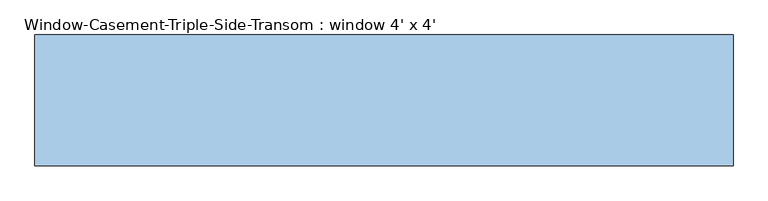
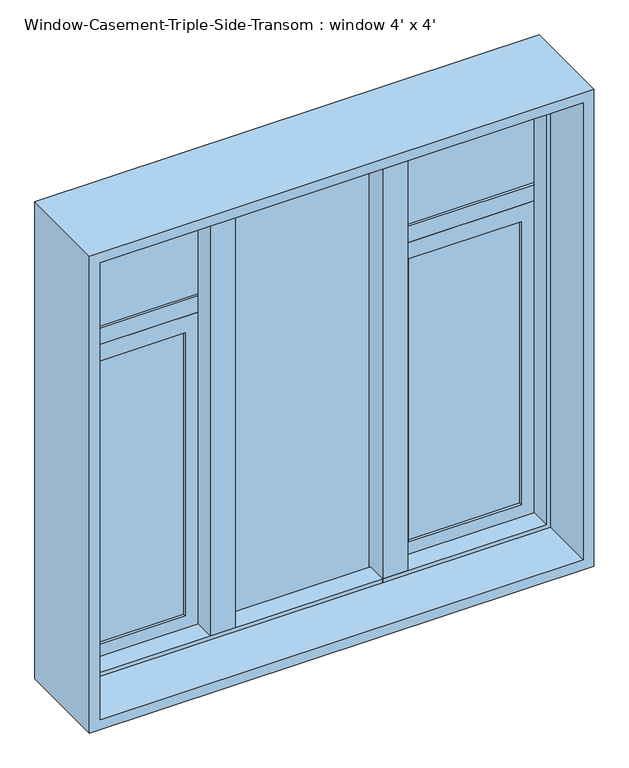
"""IFC4 building model written with IfcOpenShell, lengths in millimetres: window geometry, Window-Casement-Triple-Side-Transom : window 4' x 4'."""

from ifc_helpers import new_model, si_unit, frame, origin, place, context, project, spatial, polyline, outline, extrude, faceted_brep, source, transform, mapped, element, save


def window_casement_triple_side_transom_window_4_x_4_fd24aed3(model_context):
    return source(origin(), model_context, "Body", "SolidModel", [
        faceted_brep([(-584.2, 73.025, 2108.2), (-584.2, 114.3, 2108.2), (584.2, 114.3, 2108.2), (584.2, 73.025, 2108.2), (-574.0796875, 22.225, 2098.0796875), (-574.0796875, 73.025, 2098.0796875), (574.0796875, 73.025, 2098.0796875), (574.0796875, 22.225, 2098.0796875), (-584.2, -114.3, 2108.2), (-584.2, 22.225, 2108.2), (584.2, 22.225, 2108.2), (584.2, -114.3, 2108.2), (-609.6, 114.3, 2133.6), (-609.6, -114.3, 2133.6), (609.6, -114.3, 2133.6), (609.6, 114.3, 2133.6), (584.2, 114.3, 939.8), (584.2, 73.025, 939.8), (574.0796875, 73.025, 949.9203125), (574.0796875, 22.225, 949.9203125), (584.2, 22.225, 939.8), (584.2, -114.3, 939.8), (609.6, -114.3, 914.4), (609.6, 114.3, 914.4), (-584.2, 114.3, 939.8), (-584.2, 73.025, 939.8), (-574.0796875, 73.025, 949.9203125), (-574.0796875, 22.225, 949.9203125), (-584.2, 22.225, 939.8), (-584.2, -114.3, 939.8), (-609.6, -114.3, 914.4), (-609.6, 114.3, 914.4)], [[[0, 1, 2, 3]], [[4, 5, 6, 7]], [[8, 9, 10, 11]], [[12, 13, 14, 15]], [[3, 2, 16, 17]], [[7, 6, 18, 19]], [[11, 10, 20, 21]], [[15, 14, 22, 23]], [[17, 16, 24, 25]], [[19, 18, 26, 27]], [[21, 20, 28, 29]], [[23, 22, 30, 31]], [[25, 24, 1, 0]], [[3, 17, 25, 0], [5, 26, 18, 6]], [[27, 26, 5, 4]], [[9, 28, 20, 10], [7, 19, 27, 4]], [[29, 28, 9, 8]], [[13, 30, 22, 14], [11, 21, 29, 8]], [[31, 30, 13, 12]], [[15, 23, 31, 12], [1, 24, 16, 2]]]),
        extrude(outline(polyline([(-177.8, 111.125), (-177.8, 22.225), (-238.7203125, 22.225), (-238.7203125, 73.025), (-228.6, 73.025), (-228.6, 111.125), (-177.8, 111.125)])), frame((0.0, 0.0, 939.8), z_axis=(0.0, 0.0, 1.0), x_axis=(1.0, 0.0, 0.0)), (0.0, 0.0, 1.0), 1168.4),
        extrude(outline(polyline([(228.6, 111.125), (228.6, 73.025), (238.7203125, 73.025), (238.7203125, 22.225), (177.8, 22.225), (177.8, 111.125), (228.6, 111.125)])), frame((0.0, 0.0, 939.8), z_axis=(0.0, 0.0, 1.0), x_axis=(1.0, 0.0, 0.0)), (0.0, 0.0, 1.0), 1168.4),
        extrude(outline(polyline([(1746.9048438, 228.6), (939.8, 228.6), (939.8, 584.2), (1746.9048438, 584.2), (1746.9048438, 228.6)]), holes=[polyline([(1705.0345313, 542.3296875), (981.6703125, 542.3296875), (981.6703125, 270.4703125), (1705.0345313, 270.4703125), (1705.0345313, 542.3296875)])]), frame((0.0, 73.025, 0.0), z_axis=(0.0, 1.0, 0.0), x_axis=(0.0, 0.0, 1.0)), (0.0, 0.0, 1.0), 31.75),
        extrude(outline(polyline([(1746.9048438, -584.2), (939.8, -584.2), (939.8, -228.6), (1746.9048438, -228.6), (1746.9048438, -584.2)]), holes=[polyline([(1705.0345313, -270.4703125), (981.6703125, -270.4703125), (981.6703125, -542.3296875), (1705.0345313, -542.3296875), (1705.0345313, -270.4703125)])]), frame((0.0, 73.025, 0.0), z_axis=(0.0, 1.0, 0.0), x_axis=(0.0, 0.0, 1.0)), (0.0, 0.0, 1.0), 31.75),
        extrude(outline(polyline([(-270.4703125, 98.425), (-270.4703125, 92.075), (-542.3296875, 92.075), (-542.3296875, 98.425), (-270.4703125, 98.425)])), frame((0.0, 0.0, 981.6703125), z_axis=(0.0, 0.0, 1.0), x_axis=(1.0, 0.0, 0.0)), (0.0, 0.0, 1.0), 723.3642188),
        extrude(outline(polyline([(-270.4703125, 85.725), (-270.4703125, 79.375), (-542.3296875, 79.375), (-542.3296875, 85.725), (-270.4703125, 85.725)])), frame((0.0, 0.0, 981.6703125), z_axis=(0.0, 0.0, 1.0), x_axis=(1.0, 0.0, 0.0)), (0.0, 0.0, 1.0), 723.3642188),
        extrude(outline(polyline([(542.3296875, 98.425), (542.3296875, 92.075), (270.4703125, 92.075), (270.4703125, 98.425), (542.3296875, 98.425)])), frame((0.0, 0.0, 981.6703125), z_axis=(0.0, 0.0, 1.0), x_axis=(1.0, 0.0, 0.0)), (0.0, 0.0, 1.0), 723.3642188),
        extrude(outline(polyline([(542.3296875, 85.725), (542.3296875, 79.375), (270.4703125, 79.375), (270.4703125, 85.725), (542.3296875, 85.725)])), frame((0.0, 0.0, 981.6703125), z_axis=(0.0, 0.0, 1.0), x_axis=(1.0, 0.0, 0.0)), (0.0, 0.0, 1.0), 723.3642188),
        extrude(outline(polyline([(584.2, 104.775), (584.2, 73.025), (228.6, 73.025), (228.6, 104.775), (584.2, 104.775)])), frame((0.0, 0.0, 1746.9048438), z_axis=(0.0, 0.0, 1.0), x_axis=(1.0, 0.0, 0.0)), (0.0, 0.0, 1.0), 41.8703125),
        extrude(outline(polyline([(177.8, 98.425), (177.8, 92.075), (-177.8, 92.075), (-177.8, 98.425), (177.8, 98.425)])), frame((0.0, 0.0, 939.8), z_axis=(0.0, 0.0, 1.0), x_axis=(1.0, 0.0, 0.0)), (0.0, 0.0, 1.0), 1168.4),
        extrude(outline(polyline([(177.8, 85.725), (177.8, 79.375), (-177.8, 79.375), (-177.8, 85.725), (177.8, 85.725)])), frame((0.0, 0.0, 939.8), z_axis=(0.0, 0.0, 1.0), x_axis=(1.0, 0.0, 0.0)), (0.0, 0.0, 1.0), 1168.4),
        extrude(outline(polyline([(-228.6, 104.775), (-228.6, 73.025), (-584.2, 73.025), (-584.2, 104.775), (-228.6, 104.775)])), frame((0.0, 0.0, 1746.9048438), z_axis=(0.0, 0.0, 1.0), x_axis=(1.0, 0.0, 0.0)), (0.0, 0.0, 1.0), 41.8703125),
        extrude(outline(polyline([(-228.6, 98.425), (-228.6, 92.075), (-584.2, 92.075), (-584.2, 98.425), (-228.6, 98.425)])), frame((0.0, 0.0, 1788.7751562), z_axis=(0.0, 0.0, 1.0), x_axis=(1.0, 0.0, 0.0)), (0.0, 0.0, 1.0), 319.4248438),
        extrude(outline(polyline([(-228.6, 85.725), (-228.6, 79.375), (-584.2, 79.375), (-584.2, 85.725), (-228.6, 85.725)])), frame((0.0, 0.0, 1788.7751562), z_axis=(0.0, 0.0, 1.0), x_axis=(1.0, 0.0, 0.0)), (0.0, 0.0, 1.0), 319.4248438),
        extrude(outline(polyline([(584.2, 98.425), (584.2, 92.075), (228.6, 92.075), (228.6, 98.425), (584.2, 98.425)])), frame((0.0, 0.0, 1788.7751562), z_axis=(0.0, 0.0, 1.0), x_axis=(1.0, 0.0, 0.0)), (0.0, 0.0, 1.0), 319.4248438),
        extrude(outline(polyline([(584.2, 85.725), (584.2, 79.375), (228.6, 79.375), (228.6, 85.725), (584.2, 85.725)])), frame((0.0, 0.0, 1788.7751562), z_axis=(0.0, 0.0, 1.0), x_axis=(1.0, 0.0, 0.0)), (0.0, 0.0, 1.0), 319.4248438),
    ])


if __name__ == "__main__":
    model = new_model("IFC4")
    model_context = context("Model", 3, world=origin())
    ifc_project = project(units=[si_unit("LENGTHUNIT", "METRE", prefix="MILLI")], contexts=[model_context])
    site = spatial("IfcSite", under=ifc_project)
    building = spatial("IfcBuilding", under=site)
    placement = place(None, origin())
    window_casement_triple_side_transom_window_4_x_4_shape = window_casement_triple_side_transom_window_4_x_4_fd24aed3(model_context)
    element("IfcWindow", 1, ObjectType="Window-Casement-Triple-Side-Transom : window 4' x 4'", at=placement, inside=building, context=model_context, shape_type="MappedRepresentation", body=[
        mapped(window_casement_triple_side_transom_window_4_x_4_shape, transform((0.0, 0.0, 0.0), x_axis=(1.0, 0.0, 0.0), y_axis=(0.0, 1.0, 0.0), z_axis=(0.0, 0.0, 1.0))),
    ])
    save(model, "model.ifc")

# Revit data of these elements
# Type "Window-Casement-Triple-Side-Transom : window 4' x 4'"
#   Type Mark = "22"
#   Fire Rating = "0.5h"
#   Assembly Code = "B2020100"
#   Analytic Construction = "Double glazing - domestic"
#   Window Width = 1' - 4"
#   Window Inset [instance default] = 0' - 0 5/8"
#   Wall Thickness [instance default] = 0' - 6"
#   Visual Light Transmittance = 0.81
#   Transom Height Ratio = 0.3
#   Thermal Resistance (R) = 1.8146 (h·ft²·°F)/BTU
#   Solar Heat Gain Coefficient = 0.76
#   Rough Width = 4' - 0 1/2"
#   Rough Height = 4' - 0 1/2"
#   Open Window Height = 2' - 9.6"
#   Heat Transfer Coefficient (U) = 0.5511 BTU/(h·ft²·°F)
#   Height = 4' - 0"
#   Transom Height = 1' - 2.4"
#   Frame Gap 3 [instance default] = 0' - 1 83/128"
#   Frame Gap 2 [instance default] = 0' - 0 5/8"
#   Frame Gap 1 = 0' - 1 51/128"
#   Default Sill Height = 3' - 0"
#   Width = 4' - 0"
#   Frame Material = Metal - Aluminum
#   Glass Panel Material = Glass
#   Wall Closure = (empty or 0)
# Element 1 (IfcWindow, "Window-Casement-Triple-Side-Transom : window 4' x 4'")
#   Wall Thickness = 0' - 9"
#   Materials on its faces: "Metal - Aluminum", "Glass"
# Materials
#   "Metal - Aluminum": class "Metal", colour RGB 247 247 247, transparency 0
#   "Glass": class "Glass", colour RGB 0 128 192, transparency 0.75, Description = "Soda Lime Glass", Cost = 0
